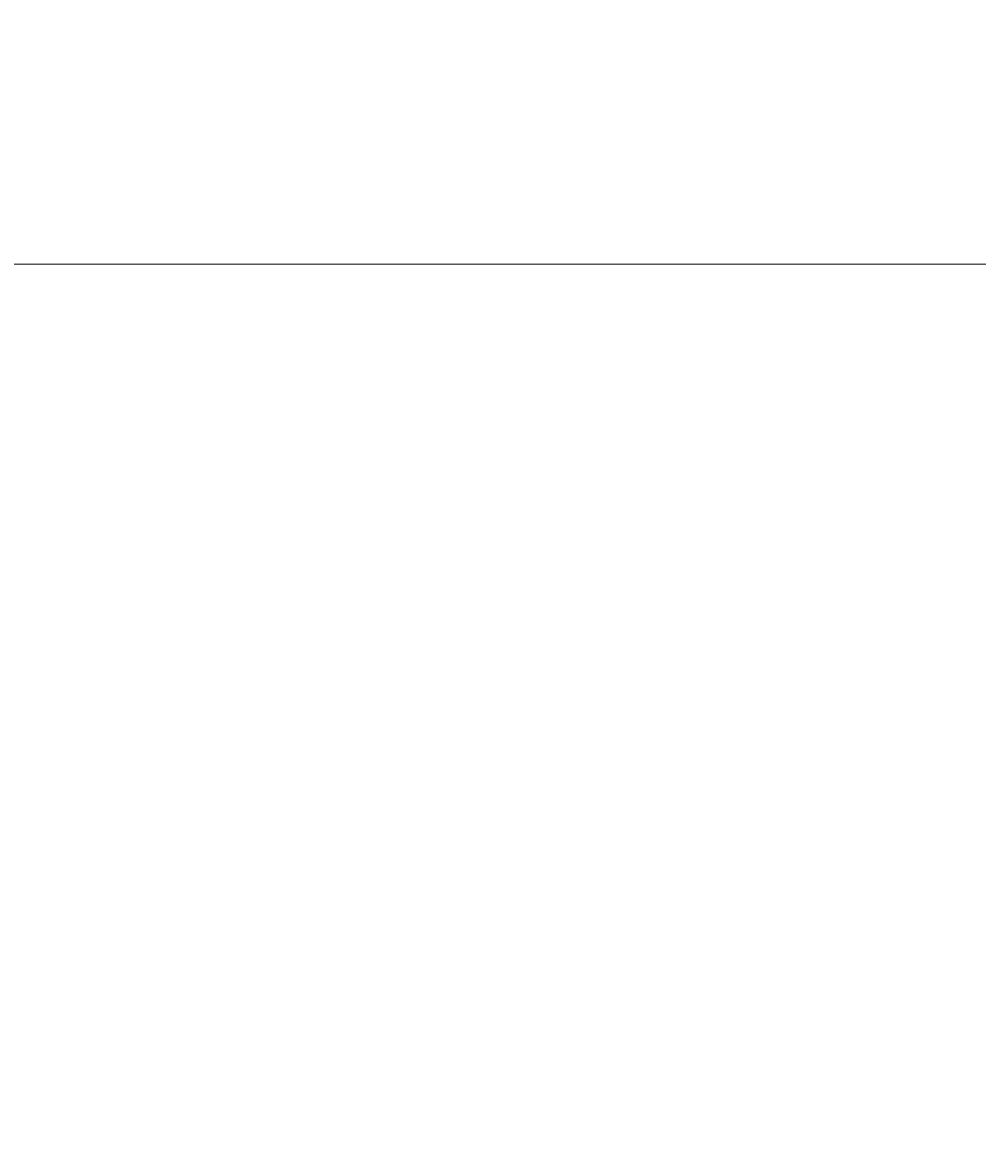
# Model space of a CAD drawing. Units: inches. Extents: x 412 to 584, y 208 to 437.
# Tile 13 of 28: x 516 to 539, y 288 to 315. Entities that reach past the tile are written whole.
import ezdxf

# ---------------------------------------------------------------- set-up
doc = ezdxf.new("R2010")
doc.units = ezdxf.units.IN
doc.header["$MEASUREMENT"] = 0
doc.layers.add('A-ANNO-DIMS', color=2, linetype='Continuous', lineweight=18)
doc.layers.add('E-ENCL', color=8, linetype='Continuous', lineweight=18)
doc.styles.get("Standard").update_dxf_attribs({"font": 'arial.ttf'})
doc.dimstyles.get("Standard").update_dxf_attribs({"dimtxt": 0.18, "dimasz": 0.18, "dimexe": 0.18, "dimexo": 0.0625, "dimgap": 0.09, "dimtad": 0, "dimtih": 1, "dimtoh": 1, "dimdec": 4, "dimzin": 0, "dimdsep": 46, "dimtxsty": 'Standard', "dimcen": 0.09, "dimadec": 0, "dimazin": 0, "dimtfac": 1, "dimtdec": 4, "dimtofl": 0, "dimtmove": 0, "dimatfit": 3, "dimfxl": 1, "dimtolj": 1, "dimtzin": 0, "dimarcsym": 0})

# ---------------------------------------------------------------- blocks, each defined once
blk = doc.blocks.new('*D17')
at = {"layer": 'A-ANNO-DIMS', "color": 0, "lineweight": -2, "transparency": 16777216}
for p, q in [((497.715, 426.185), (583.674, 426.185)), ((583.494, 426.005), (583.494, 323.031)), ((583.494, 219.693), (583.494, 322.667)), ((550.198, 219.513), (583.674, 219.513))]:
    blk.add_line(p, q, dxfattribs=at)
at = {"layer": 'A-ANNO-DIMS', "color": 0, "transparency": 16777216}
for points in [[(583.464, 426.005), (583.524, 426.005), (583.494, 426.185)], [(583.464, 219.693), (583.524, 219.693), (583.494, 219.513)]]:
    blk.add_solid(points, dxfattribs=at)
at = {"layer": 'Defpoints', "color": 0, "transparency": 16777216}
for p in [(497.652, 426.185), (550.135, 219.513), (583.494, 219.513)]:
    blk.add_point(p, dxfattribs=at)
at = {"layer": 'A-ANNO-DIMS', "color": 0, "transparency": 16777216, "insert": (583.494, 322.849), "char_height": 0.18, "attachment_point": 5}
blk.add_mtext('\\A1;206.67', dxfattribs=at)
blk = doc.blocks.new('*D28')
at = {"layer": 'A-ANNO-DIMS', "color": 0, "lineweight": -2, "transparency": 16777216}
for p, q in [((450.562, 256.635), (450.562, 437.465)), ((450.742, 437.285), (502.724, 437.285)), ((555.616, 437.285), (503.634, 437.285)), ((555.796, 256.635), (555.796, 437.465))]:
    blk.add_line(p, q, dxfattribs=at)
at = {"layer": 'A-ANNO-DIMS', "color": 0, "transparency": 16777216}
for points in [[(450.742, 437.315), (450.742, 437.255), (450.562, 437.285)], [(555.616, 437.315), (555.616, 437.255), (555.796, 437.285)]]:
    blk.add_solid(points, dxfattribs=at)
at = {"layer": 'Defpoints', "color": 0, "transparency": 16777216}
for p in [(555.796, 437.285), (450.562, 256.573), (555.796, 256.573)]:
    blk.add_point(p, dxfattribs=at)
at = {"layer": 'A-ANNO-DIMS', "color": 0, "transparency": 16777216, "insert": (503.179, 437.285), "char_height": 0.18, "attachment_point": 5}
blk.add_mtext('\\A1;105.23', dxfattribs=at)

msp = doc.modelspace()

# ---------------------------------------------------------------- linework, layer by layer
at = {"layer": 'E-ENCL'}
msp.add_lwpolyline([(423.5562, 309.3773), (572.3937, 309.3773), (572.3937, 225.5881), (423.5562, 225.5881)], close=True, dxfattribs=at)

# ---------------------------------------------------------------- dimensions: what is measured, and where the dimension line sits
at = {"layer": 'A-ANNO-DIMS'}
dim = msp.add_linear_dim(base=(555.7959, 437.2847), p1=(450.562, 256.5729), p2=(555.7959, 256.5729), dimstyle='Standard', override={"dimdec": 2, "dimlfac": 1, "dimrnd": 0, "dimzin": 0, "dimdsep": 46, "dimlunit": 2}, dxfattribs=at)
dim.commit()
dim.dimension.update_dxf_attribs({"geometry": '*D28', "text_midpoint": (503.1789, 437.2847)})
dim = msp.add_linear_dim(base=(583.4937, 219.5133), p1=(497.6523, 426.1847), p2=(550.1351, 219.5133), angle=90, dimstyle='Standard', override={"dimdec": 2, "dimlfac": 1, "dimrnd": 0, "dimzin": 0, "dimdsep": 46, "dimlunit": 2}, dxfattribs=at)
dim.commit()
dim.dimension.update_dxf_attribs({"geometry": '*D17', "text_midpoint": (583.4937, 322.849)})

doc.saveas('drawing.dxf')
